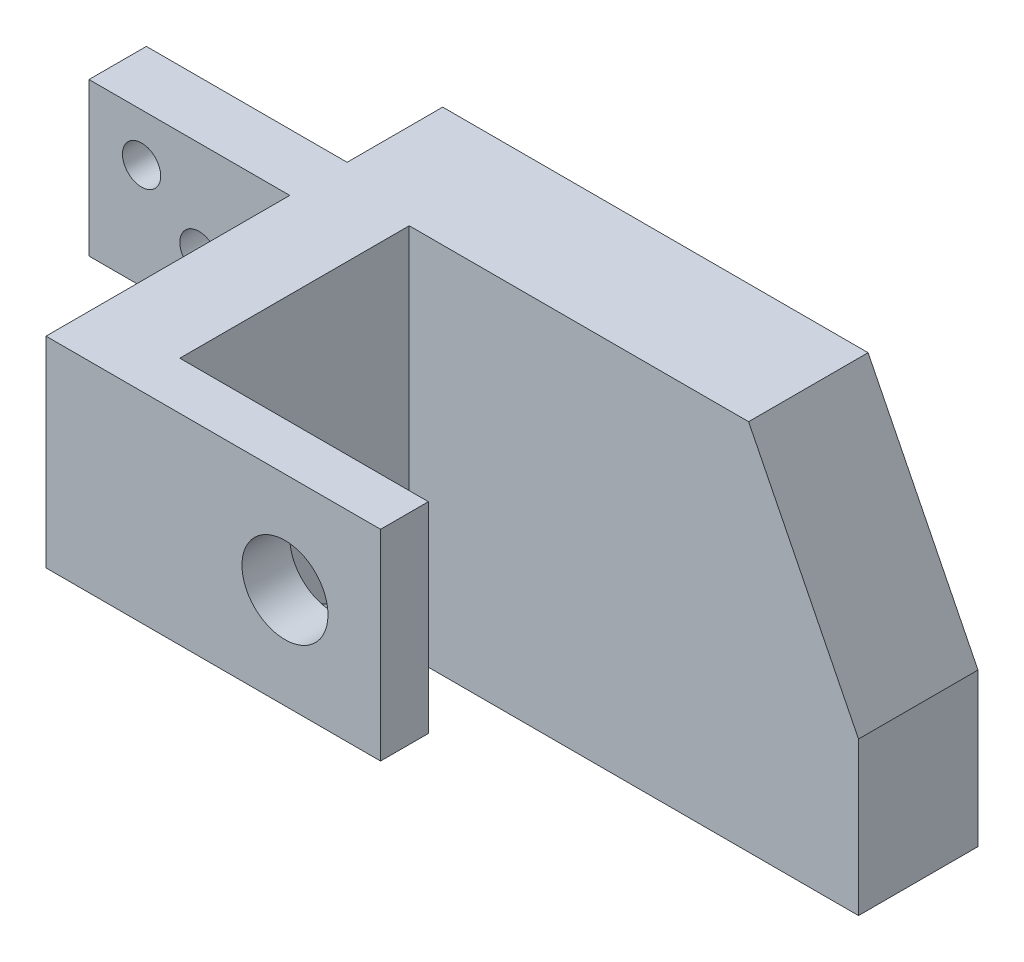
ISO-10303-21;
HEADER;
FILE_DESCRIPTION(('STEP AP214'),'2;1');
FILE_NAME('part.step','',(''),(''),'','','');
FILE_SCHEMA(('AUTOMOTIVE_DESIGN { 1 0 10303 214 1 1 1 1 }'));
ENDSEC;
DATA;
#1=APPLICATION_CONTEXT('core data for automotive mechanical design processes');
#2=APPLICATION_PROTOCOL_DEFINITION('international standard','automotive_design',2000,#1);
#3=PRODUCT_CONTEXT('',#1,'mechanical');
#4=PRODUCT('Part','Part','',(#3));
#5=PRODUCT_RELATED_PRODUCT_CATEGORY('part','',(#4));
#6=PRODUCT_DEFINITION_FORMATION('','',#4);
#7=PRODUCT_DEFINITION_CONTEXT('part definition',#1,'design');
#8=PRODUCT_DEFINITION('design','',#6,#7);
#9=PRODUCT_DEFINITION_SHAPE('','',#8);
#10=(LENGTH_UNIT() NAMED_UNIT(*) SI_UNIT(.MILLI.,.METRE.));
#11=(NAMED_UNIT(*) PLANE_ANGLE_UNIT() SI_UNIT($,.RADIAN.));
#12=(NAMED_UNIT(*) SI_UNIT($,.STERADIAN.) SOLID_ANGLE_UNIT());
#13=UNCERTAINTY_MEASURE_WITH_UNIT(LENGTH_MEASURE(1.E-05),#10,'distance_accuracy_value','');
#14=(GEOMETRIC_REPRESENTATION_CONTEXT(3) GLOBAL_UNCERTAINTY_ASSIGNED_CONTEXT((#13)) GLOBAL_UNIT_ASSIGNED_CONTEXT((#10,
#11,#12)) REPRESENTATION_CONTEXT('',''));
#15=CARTESIAN_POINT('',(0.,0.,0.));
#16=DIRECTION('',(0.,0.,1.));
#17=DIRECTION('',(1.,0.,0.));
#18=AXIS2_PLACEMENT_3D('',#15,#16,#17);
#19=CARTESIAN_POINT('',(0.,0.,25.));
#20=DIRECTION('',(1.,0.,0.));
#21=DIRECTION('',(0.,0.,-1.));
#22=AXIS2_PLACEMENT_3D('',#19,#20,#21);
#23=PLANE('',#22);
#24=DIRECTION('',(0.,-1.,0.));
#25=VECTOR('',#24,1.);
#26=CARTESIAN_POINT('',(0.,0.,25.));
#27=LINE('',#26,#25);
#28=CARTESIAN_POINT('',(0.,7.99999999999999,25.));
#29=VERTEX_POINT('',#28);
#30=CARTESIAN_POINT('',(0.,0.,25.));
#31=VERTEX_POINT('',#30);
#32=EDGE_CURVE('E254',#29,#31,#27,.T.);
#33=ORIENTED_EDGE('',*,*,#32,.F.);
#34=DIRECTION('',(0.,0.503871025524086,0.863778900898433));
#35=VECTOR('',#34,1.);
#36=CARTESIAN_POINT('',(0.,7.99999999999999,25.));
#37=LINE('',#36,#35);
#38=CARTESIAN_POINT('',(0.,36.,73.));
#39=VERTEX_POINT('',#38);
#40=EDGE_CURVE('E177',#29,#39,#37,.T.);
#41=ORIENTED_EDGE('',*,*,#40,.T.);
#42=DIRECTION('',(0.,0.,1.));
#43=VECTOR('',#42,1.);
#44=CARTESIAN_POINT('',(0.,36.,83.));
#45=LINE('',#44,#43);
#46=CARTESIAN_POINT('',(0.,36.,83.));
#47=VERTEX_POINT('',#46);
#48=EDGE_CURVE('E175',#39,#47,#45,.T.);
#49=ORIENTED_EDGE('',*,*,#48,.T.);
#50=DIRECTION('',(0.,1.,0.));
#51=VECTOR('',#50,1.);
#52=CARTESIAN_POINT('',(0.,78.,83.));
#53=LINE('',#52,#51);
#54=CARTESIAN_POINT('',(0.,78.,83.));
#55=VERTEX_POINT('',#54);
#56=EDGE_CURVE('E245',#47,#55,#53,.T.);
#57=ORIENTED_EDGE('',*,*,#56,.T.);
#58=DIRECTION('',(0.,0.,-1.));
#59=VECTOR('',#58,1.);
#60=CARTESIAN_POINT('',(0.,78.,25.));
#61=LINE('',#60,#59);
#62=CARTESIAN_POINT('',(0.,78.,32.));
#63=VERTEX_POINT('',#62);
#64=EDGE_CURVE('E273',#55,#63,#61,.T.);
#65=ORIENTED_EDGE('',*,*,#64,.T.);
#66=DIRECTION('',(0.,1.,0.));
#67=VECTOR('',#66,1.);
#68=CARTESIAN_POINT('',(0.,46.,32.));
#69=LINE('',#68,#67);
#70=CARTESIAN_POINT('',(0.,46.,32.));
#71=VERTEX_POINT('',#70);
#72=EDGE_CURVE('E218',#71,#63,#69,.T.);
#73=ORIENTED_EDGE('',*,*,#72,.F.);
#74=DIRECTION('',(0.,0.,1.));
#75=VECTOR('',#74,1.);
#76=CARTESIAN_POINT('',(0.,46.,20.));
#77=LINE('',#76,#75);
#78=CARTESIAN_POINT('',(0.,46.,20.));
#79=VERTEX_POINT('',#78);
#80=EDGE_CURVE('E223',#79,#71,#77,.T.);
#81=ORIENTED_EDGE('',*,*,#80,.F.);
#82=DIRECTION('',(0.,-1.,0.));
#83=VECTOR('',#82,1.);
#84=CARTESIAN_POINT('',(0.,78.,20.));
#85=LINE('',#84,#83);
#86=CARTESIAN_POINT('',(0.,78.,20.));
#87=VERTEX_POINT('',#86);
#88=EDGE_CURVE('E208',#87,#79,#85,.T.);
#89=ORIENTED_EDGE('',*,*,#88,.F.);
#90=CARTESIAN_POINT('',(0.,78.,0.));
#91=VERTEX_POINT('',#90);
#92=EDGE_CURVE('E264',#87,#91,#61,.T.);
#93=ORIENTED_EDGE('',*,*,#92,.T.);
#94=DIRECTION('',(0.,-1.,0.));
#95=VECTOR('',#94,1.);
#96=CARTESIAN_POINT('',(0.,0.,0.));
#97=LINE('',#96,#95);
#98=CARTESIAN_POINT('',(0.,0.,0.));
#99=VERTEX_POINT('',#98);
#100=EDGE_CURVE('E252',#91,#99,#97,.T.);
#101=ORIENTED_EDGE('',*,*,#100,.T.);
#102=DIRECTION('',(0.,0.,-1.));
#103=VECTOR('',#102,1.);
#104=CARTESIAN_POINT('',(0.,0.,25.));
#105=LINE('',#104,#103);
#106=EDGE_CURVE('E11',#31,#99,#105,.T.);
#107=ORIENTED_EDGE('',*,*,#106,.F.);
#108=EDGE_LOOP('',(#33,#41,#49,#57,#65,#73,#81,#89,#93,#101,#107));
#109=FACE_BOUND('',#108,.T.);
#110=ADVANCED_FACE('F44',(#109),#23,.F.);
#111=CARTESIAN_POINT('',(0.,0.,25.));
#112=DIRECTION('',(0.,1.,0.));
#113=DIRECTION('',(0.,0.,1.));
#114=AXIS2_PLACEMENT_3D('',#111,#112,#113);
#115=PLANE('',#114);
#116=DIRECTION('',(1.,0.,0.));
#117=VECTOR('',#116,1.);
#118=CARTESIAN_POINT('',(0.,0.,0.));
#119=LINE('',#118,#117);
#120=CARTESIAN_POINT('',(112.,0.,0.));
#121=VERTEX_POINT('',#120);
#122=EDGE_CURVE('E270',#99,#121,#119,.T.);
#123=ORIENTED_EDGE('',*,*,#122,.T.);
#124=DIRECTION('',(0.,0.,-1.));
#125=VECTOR('',#124,1.);
#126=CARTESIAN_POINT('',(112.,0.,25.));
#127=LINE('',#126,#125);
#128=CARTESIAN_POINT('',(112.,0.,25.));
#129=VERTEX_POINT('',#128);
#130=EDGE_CURVE('E55',#129,#121,#127,.T.);
#131=ORIENTED_EDGE('',*,*,#130,.F.);
#132=DIRECTION('',(1.,0.,0.));
#133=VECTOR('',#132,1.);
#134=CARTESIAN_POINT('',(0.,0.,25.));
#135=LINE('',#134,#133);
#136=EDGE_CURVE('E253',#31,#129,#135,.T.);
#137=ORIENTED_EDGE('',*,*,#136,.F.);
#138=ORIENTED_EDGE('',*,*,#106,.T.);
#139=EDGE_LOOP('',(#123,#131,#137,#138));
#140=FACE_BOUND('',#139,.T.);
#141=ADVANCED_FACE('F306',(#140),#115,.F.);
#142=CARTESIAN_POINT('',(112.,0.,25.));
#143=DIRECTION('',(-1.,0.,0.));
#144=DIRECTION('',(0.,0.,1.));
#145=AXIS2_PLACEMENT_3D('',#142,#143,#144);
#146=PLANE('',#145);
#147=DIRECTION('',(0.,1.,0.));
#148=VECTOR('',#147,1.);
#149=CARTESIAN_POINT('',(112.,0.,0.));
#150=LINE('',#149,#148);
#151=CARTESIAN_POINT('',(112.,32.,0.));
#152=VERTEX_POINT('',#151);
#153=EDGE_CURVE('E266',#121,#152,#150,.T.);
#154=ORIENTED_EDGE('',*,*,#153,.T.);
#155=DIRECTION('',(0.,0.,-1.));
#156=VECTOR('',#155,1.);
#157=CARTESIAN_POINT('',(112.,32.,25.));
#158=LINE('',#157,#156);
#159=CARTESIAN_POINT('',(112.,32.,25.));
#160=VERTEX_POINT('',#159);
#161=EDGE_CURVE('E278',#160,#152,#158,.T.);
#162=ORIENTED_EDGE('',*,*,#161,.F.);
#163=DIRECTION('',(0.,1.,0.));
#164=VECTOR('',#163,1.);
#165=CARTESIAN_POINT('',(112.,0.,25.));
#166=LINE('',#165,#164);
#167=EDGE_CURVE('E259',#129,#160,#166,.T.);
#168=ORIENTED_EDGE('',*,*,#167,.F.);
#169=ORIENTED_EDGE('',*,*,#130,.T.);
#170=EDGE_LOOP('',(#154,#162,#168,#169));
#171=FACE_BOUND('',#170,.T.);
#172=ADVANCED_FACE('F290',(#171),#146,.F.);
#173=CARTESIAN_POINT('',(89.,78.,25.));
#174=DIRECTION('',(-0.894427190999916,-0.447213595499958,0.));
#175=DIRECTION('',(0.447213595499958,-0.894427190999916,0.));
#176=AXIS2_PLACEMENT_3D('',#173,#174,#175);
#177=PLANE('',#176);
#178=DIRECTION('',(-0.447213595499958,0.894427190999916,0.));
#179=VECTOR('',#178,1.);
#180=CARTESIAN_POINT('',(89.,78.,0.));
#181=LINE('',#180,#179);
#182=CARTESIAN_POINT('',(89.,78.,0.));
#183=VERTEX_POINT('',#182);
#184=EDGE_CURVE('E272',#152,#183,#181,.T.);
#185=ORIENTED_EDGE('',*,*,#184,.T.);
#186=DIRECTION('',(0.,0.,-1.));
#187=VECTOR('',#186,1.);
#188=CARTESIAN_POINT('',(89.,78.,25.));
#189=LINE('',#188,#187);
#190=CARTESIAN_POINT('',(89.,78.,25.));
#191=VERTEX_POINT('',#190);
#192=EDGE_CURVE('E280',#191,#183,#189,.T.);
#193=ORIENTED_EDGE('',*,*,#192,.F.);
#194=DIRECTION('',(-0.447213595499958,0.894427190999916,0.));
#195=VECTOR('',#194,1.);
#196=CARTESIAN_POINT('',(89.,78.,25.));
#197=LINE('',#196,#195);
#198=EDGE_CURVE('E258',#160,#191,#197,.T.);
#199=ORIENTED_EDGE('',*,*,#198,.F.);
#200=ORIENTED_EDGE('',*,*,#161,.T.);
#201=EDGE_LOOP('',(#185,#193,#199,#200));
#202=FACE_BOUND('',#201,.T.);
#203=ADVANCED_FACE('F296',(#202),#177,.F.);
#204=CARTESIAN_POINT('',(0.,78.,25.));
#205=DIRECTION('',(0.,-1.,0.));
#206=DIRECTION('',(0.,0.,-1.));
#207=AXIS2_PLACEMENT_3D('',#204,#205,#206);
#208=PLANE('',#207);
#209=DIRECTION('',(-1.,0.,0.));
#210=VECTOR('',#209,1.);
#211=CARTESIAN_POINT('',(0.,78.,0.));
#212=LINE('',#211,#210);
#213=EDGE_CURVE('E257',#183,#91,#212,.T.);
#214=ORIENTED_EDGE('',*,*,#213,.T.);
#215=ORIENTED_EDGE('',*,*,#92,.F.);
#216=DIRECTION('',(1.,0.,0.));
#217=VECTOR('',#216,1.);
#218=CARTESIAN_POINT('',(-42.,78.,20.));
#219=LINE('',#218,#217);
#220=CARTESIAN_POINT('',(-42.,78.,20.));
#221=VERTEX_POINT('',#220);
#222=EDGE_CURVE('E238',#221,#87,#219,.T.);
#223=ORIENTED_EDGE('',*,*,#222,.F.);
#224=DIRECTION('',(0.,0.,-1.));
#225=VECTOR('',#224,1.);
#226=CARTESIAN_POINT('',(-42.,78.,32.));
#227=LINE('',#226,#225);
#228=CARTESIAN_POINT('',(-42.,78.,32.));
#229=VERTEX_POINT('',#228);
#230=EDGE_CURVE('E215',#229,#221,#227,.T.);
#231=ORIENTED_EDGE('',*,*,#230,.F.);
#232=DIRECTION('',(1.,0.,0.));
#233=VECTOR('',#232,1.);
#234=CARTESIAN_POINT('',(-42.,78.,32.));
#235=LINE('',#234,#233);
#236=EDGE_CURVE('E225',#229,#63,#235,.T.);
#237=ORIENTED_EDGE('',*,*,#236,.T.);
#238=ORIENTED_EDGE('',*,*,#64,.F.);
#239=DIRECTION('',(-1.,0.,0.));
#240=VECTOR('',#239,1.);
#241=CARTESIAN_POINT('',(18.,78.,83.));
#242=LINE('',#241,#240);
#243=CARTESIAN_POINT('',(70.,78.,83.));
#244=VERTEX_POINT('',#243);
#245=EDGE_CURVE('E247',#244,#55,#242,.T.);
#246=ORIENTED_EDGE('',*,*,#245,.F.);
#247=DIRECTION('',(0.,0.,1.));
#248=VECTOR('',#247,1.);
#249=CARTESIAN_POINT('',(70.,78.,73.));
#250=LINE('',#249,#248);
#251=CARTESIAN_POINT('',(70.,78.,73.));
#252=VERTEX_POINT('',#251);
#253=EDGE_CURVE('E210',#252,#244,#250,.T.);
#254=ORIENTED_EDGE('',*,*,#253,.F.);
#255=DIRECTION('',(-1.,0.,0.));
#256=VECTOR('',#255,1.);
#257=CARTESIAN_POINT('',(18.,78.,73.));
#258=LINE('',#257,#256);
#259=CARTESIAN_POINT('',(18.,78.,73.));
#260=VERTEX_POINT('',#259);
#261=EDGE_CURVE('E205',#252,#260,#258,.T.);
#262=ORIENTED_EDGE('',*,*,#261,.T.);
#263=DIRECTION('',(0.,0.,-1.));
#264=VECTOR('',#263,1.);
#265=CARTESIAN_POINT('',(18.,78.,25.));
#266=LINE('',#265,#264);
#267=CARTESIAN_POINT('',(18.,78.,25.));
#268=VERTEX_POINT('',#267);
#269=EDGE_CURVE('E155',#260,#268,#266,.T.);
#270=ORIENTED_EDGE('',*,*,#269,.T.);
#271=DIRECTION('',(-1.,0.,0.));
#272=VECTOR('',#271,1.);
#273=CARTESIAN_POINT('',(0.,78.,25.));
#274=LINE('',#273,#272);
#275=EDGE_CURVE('E265',#191,#268,#274,.T.);
#276=ORIENTED_EDGE('',*,*,#275,.F.);
#277=ORIENTED_EDGE('',*,*,#192,.T.);
#278=EDGE_LOOP('',(#214,#215,#223,#231,#237,#238,#246,#254,#262,#270,#276,#277));
#279=FACE_BOUND('',#278,.T.);
#280=ADVANCED_FACE('F305',(#279),#208,.F.);
#281=CARTESIAN_POINT('',(0.,0.,25.));
#282=DIRECTION('',(0.,0.,-1.));
#283=DIRECTION('',(-1.,0.,0.));
#284=AXIS2_PLACEMENT_3D('',#281,#282,#283);
#285=PLANE('',#284);
#286=DIRECTION('',(0.,-1.,0.));
#287=VECTOR('',#286,1.);
#288=CARTESIAN_POINT('',(18.,36.,25.));
#289=LINE('',#288,#287);
#290=CARTESIAN_POINT('',(18.,7.99999999999999,25.));
#291=VERTEX_POINT('',#290);
#292=EDGE_CURVE('E56',#268,#291,#289,.T.);
#293=ORIENTED_EDGE('',*,*,#292,.T.);
#294=DIRECTION('',(-1.,0.,0.));
#295=VECTOR('',#294,1.);
#296=CARTESIAN_POINT('',(18.,7.99999999999999,25.));
#297=LINE('',#296,#295);
#298=EDGE_CURVE('E64',#291,#29,#297,.T.);
#299=ORIENTED_EDGE('',*,*,#298,.T.);
#300=ORIENTED_EDGE('',*,*,#32,.T.);
#301=ORIENTED_EDGE('',*,*,#136,.T.);
#302=ORIENTED_EDGE('',*,*,#167,.T.);
#303=ORIENTED_EDGE('',*,*,#198,.T.);
#304=ORIENTED_EDGE('',*,*,#275,.T.);
#305=EDGE_LOOP('',(#293,#299,#300,#301,#302,#303,#304));
#306=FACE_BOUND('',#305,.T.);
#307=ADVANCED_FACE('F302',(#306),#285,.F.);
#308=CARTESIAN_POINT('',(0.,0.,0.));
#309=DIRECTION('',(0.,0.,-1.));
#310=DIRECTION('',(-1.,0.,0.));
#311=AXIS2_PLACEMENT_3D('',#308,#309,#310);
#312=PLANE('',#311);
#313=ORIENTED_EDGE('',*,*,#100,.F.);
#314=ORIENTED_EDGE('',*,*,#213,.F.);
#315=ORIENTED_EDGE('',*,*,#184,.F.);
#316=ORIENTED_EDGE('',*,*,#153,.F.);
#317=ORIENTED_EDGE('',*,*,#122,.F.);
#318=EDGE_LOOP('',(#313,#314,#315,#316,#317));
#319=FACE_BOUND('',#318,.T.);
#320=ADVANCED_FACE('F295',(#319),#312,.T.);
#321=CARTESIAN_POINT('',(18.,78.,83.));
#322=DIRECTION('',(0.,0.,1.));
#323=DIRECTION('',(1.,0.,0.));
#324=AXIS2_PLACEMENT_3D('',#321,#322,#323);
#325=PLANE('',#324);
#326=CARTESIAN_POINT('',(50.,57.,83.));
#327=DIRECTION('',(0.,0.,1.));
#328=DIRECTION('',(1.,0.,0.));
#329=AXIS2_PLACEMENT_3D('',#326,#327,#328);
#330=CIRCLE('',#329,9.);
#331=CARTESIAN_POINT('',(59.,57.,83.));
#332=VERTEX_POINT('',#331);
#333=EDGE_CURVE('E190',#332,#332,#330,.T.);
#334=ORIENTED_EDGE('',*,*,#333,.F.);
#335=EDGE_LOOP('',(#334));
#336=FACE_BOUND('',#335,.T.);
#337=ORIENTED_EDGE('',*,*,#56,.F.);
#338=DIRECTION('',(-1.,0.,0.));
#339=VECTOR('',#338,1.);
#340=CARTESIAN_POINT('',(18.,36.,83.));
#341=LINE('',#340,#339);
#342=CARTESIAN_POINT('',(70.,36.,83.));
#343=VERTEX_POINT('',#342);
#344=EDGE_CURVE('E242',#343,#47,#341,.T.);
#345=ORIENTED_EDGE('',*,*,#344,.F.);
#346=DIRECTION('',(0.,1.,0.));
#347=VECTOR('',#346,1.);
#348=CARTESIAN_POINT('',(70.,78.,83.));
#349=LINE('',#348,#347);
#350=EDGE_CURVE('E160',#343,#244,#349,.T.);
#351=ORIENTED_EDGE('',*,*,#350,.T.);
#352=ORIENTED_EDGE('',*,*,#245,.T.);
#353=EDGE_LOOP('',(#337,#345,#351,#352));
#354=FACE_BOUND('',#353,.T.);
#355=ADVANCED_FACE('F346',(#336,#354),#325,.T.);
#356=CARTESIAN_POINT('',(18.,36.,83.));
#357=DIRECTION('',(0.,-1.,0.));
#358=DIRECTION('',(0.,0.,-1.));
#359=AXIS2_PLACEMENT_3D('',#356,#357,#358);
#360=PLANE('',#359);
#361=DIRECTION('',(-1.,0.,0.));
#362=VECTOR('',#361,1.);
#363=CARTESIAN_POINT('',(18.,36.,73.));
#364=LINE('',#363,#362);
#365=CARTESIAN_POINT('',(18.,36.,73.));
#366=VERTEX_POINT('',#365);
#367=EDGE_CURVE('E169',#366,#39,#364,.T.);
#368=ORIENTED_EDGE('',*,*,#367,.F.);
#369=DIRECTION('',(1.,0.,0.));
#370=VECTOR('',#369,1.);
#371=CARTESIAN_POINT('',(70.,36.,73.));
#372=LINE('',#371,#370);
#373=CARTESIAN_POINT('',(70.,36.,73.));
#374=VERTEX_POINT('',#373);
#375=EDGE_CURVE('E157',#366,#374,#372,.T.);
#376=ORIENTED_EDGE('',*,*,#375,.T.);
#377=DIRECTION('',(0.,0.,1.));
#378=VECTOR('',#377,1.);
#379=CARTESIAN_POINT('',(70.,36.,73.));
#380=LINE('',#379,#378);
#381=EDGE_CURVE('E201',#374,#343,#380,.T.);
#382=ORIENTED_EDGE('',*,*,#381,.T.);
#383=ORIENTED_EDGE('',*,*,#344,.T.);
#384=ORIENTED_EDGE('',*,*,#48,.F.);
#385=EDGE_LOOP('',(#368,#376,#382,#383,#384));
#386=FACE_BOUND('',#385,.T.);
#387=ADVANCED_FACE('F167',(#386),#360,.T.);
#388=CARTESIAN_POINT('',(18.,0.,0.));
#389=DIRECTION('',(1.,0.,0.));
#390=DIRECTION('',(0.,0.,-1.));
#391=AXIS2_PLACEMENT_3D('',#388,#389,#390);
#392=PLANE('',#391);
#393=DIRECTION('',(0.,-1.,0.));
#394=VECTOR('',#393,1.);
#395=CARTESIAN_POINT('',(18.,36.,73.));
#396=LINE('',#395,#394);
#397=EDGE_CURVE('E150',#260,#366,#396,.T.);
#398=ORIENTED_EDGE('',*,*,#397,.T.);
#399=DIRECTION('',(0.,0.503871025524086,0.863778900898433));
#400=VECTOR('',#399,1.);
#401=CARTESIAN_POINT('',(18.,7.99999999999999,25.));
#402=LINE('',#401,#400);
#403=EDGE_CURVE('E153',#291,#366,#402,.T.);
#404=ORIENTED_EDGE('',*,*,#403,.F.);
#405=ORIENTED_EDGE('',*,*,#292,.F.);
#406=ORIENTED_EDGE('',*,*,#269,.F.);
#407=EDGE_LOOP('',(#398,#404,#405,#406));
#408=FACE_BOUND('',#407,.T.);
#409=ADVANCED_FACE('F146',(#408),#392,.T.);
#410=CARTESIAN_POINT('',(-42.,78.,20.));
#411=DIRECTION('',(0.,0.,1.));
#412=DIRECTION('',(1.,0.,0.));
#413=AXIS2_PLACEMENT_3D('',#410,#411,#412);
#414=PLANE('',#413);
#415=CARTESIAN_POINT('',(-31.,68.,20.));
#416=DIRECTION('',(0.,0.,1.));
#417=DIRECTION('',(1.,0.,0.));
#418=AXIS2_PLACEMENT_3D('',#415,#416,#417);
#419=CIRCLE('',#418,4.);
#420=CARTESIAN_POINT('',(-27.,68.,20.));
#421=VERTEX_POINT('',#420);
#422=EDGE_CURVE('E183',#421,#421,#419,.T.);
#423=ORIENTED_EDGE('',*,*,#422,.T.);
#424=EDGE_LOOP('',(#423));
#425=FACE_BOUND('',#424,.T.);
#426=CARTESIAN_POINT('',(-19.,58.,20.));
#427=DIRECTION('',(0.,0.,1.));
#428=DIRECTION('',(1.,0.,0.));
#429=AXIS2_PLACEMENT_3D('',#426,#427,#428);
#430=CIRCLE('',#429,4.);
#431=CARTESIAN_POINT('',(-15.,58.,20.));
#432=VERTEX_POINT('',#431);
#433=EDGE_CURVE('E192',#432,#432,#430,.T.);
#434=ORIENTED_EDGE('',*,*,#433,.T.);
#435=EDGE_LOOP('',(#434));
#436=FACE_BOUND('',#435,.T.);
#437=ORIENTED_EDGE('',*,*,#88,.T.);
#438=DIRECTION('',(1.,0.,0.));
#439=VECTOR('',#438,1.);
#440=CARTESIAN_POINT('',(-42.,46.,20.));
#441=LINE('',#440,#439);
#442=CARTESIAN_POINT('',(-42.,46.,20.));
#443=VERTEX_POINT('',#442);
#444=EDGE_CURVE('E232',#443,#79,#441,.T.);
#445=ORIENTED_EDGE('',*,*,#444,.F.);
#446=DIRECTION('',(0.,-1.,0.));
#447=VECTOR('',#446,1.);
#448=CARTESIAN_POINT('',(-42.,78.,20.));
#449=LINE('',#448,#447);
#450=EDGE_CURVE('E213',#221,#443,#449,.T.);
#451=ORIENTED_EDGE('',*,*,#450,.F.);
#452=ORIENTED_EDGE('',*,*,#222,.T.);
#453=EDGE_LOOP('',(#437,#445,#451,#452));
#454=FACE_BOUND('',#453,.T.);
#455=ADVANCED_FACE('F311',(#425,#436,#454),#414,.F.);
#456=CARTESIAN_POINT('',(-42.,46.,20.));
#457=DIRECTION('',(0.,1.,0.));
#458=DIRECTION('',(0.,0.,1.));
#459=AXIS2_PLACEMENT_3D('',#456,#457,#458);
#460=PLANE('',#459);
#461=ORIENTED_EDGE('',*,*,#80,.T.);
#462=DIRECTION('',(1.,0.,0.));
#463=VECTOR('',#462,1.);
#464=CARTESIAN_POINT('',(-42.,46.,32.));
#465=LINE('',#464,#463);
#466=CARTESIAN_POINT('',(-42.,46.,32.));
#467=VERTEX_POINT('',#466);
#468=EDGE_CURVE('E235',#467,#71,#465,.T.);
#469=ORIENTED_EDGE('',*,*,#468,.F.);
#470=DIRECTION('',(0.,0.,1.));
#471=VECTOR('',#470,1.);
#472=CARTESIAN_POINT('',(-42.,46.,20.));
#473=LINE('',#472,#471);
#474=EDGE_CURVE('E216',#443,#467,#473,.T.);
#475=ORIENTED_EDGE('',*,*,#474,.F.);
#476=ORIENTED_EDGE('',*,*,#444,.T.);
#477=EDGE_LOOP('',(#461,#469,#475,#476));
#478=FACE_BOUND('',#477,.T.);
#479=ADVANCED_FACE('F325',(#478),#460,.F.);
#480=CARTESIAN_POINT('',(-42.,46.,32.));
#481=DIRECTION('',(0.,0.,-1.));
#482=DIRECTION('',(0.,1.,0.));
#483=AXIS2_PLACEMENT_3D('',#480,#481,#482);
#484=PLANE('',#483);
#485=CARTESIAN_POINT('',(-31.,68.,32.));
#486=DIRECTION('',(0.,0.,1.));
#487=DIRECTION('',(1.,0.,0.));
#488=AXIS2_PLACEMENT_3D('',#485,#486,#487);
#489=CIRCLE('',#488,4.);
#490=CARTESIAN_POINT('',(-27.,68.,32.));
#491=VERTEX_POINT('',#490);
#492=EDGE_CURVE('E189',#491,#491,#489,.T.);
#493=ORIENTED_EDGE('',*,*,#492,.F.);
#494=EDGE_LOOP('',(#493));
#495=FACE_BOUND('',#494,.T.);
#496=CARTESIAN_POINT('',(-19.,58.,32.));
#497=DIRECTION('',(0.,0.,1.));
#498=DIRECTION('',(1.,0.,0.));
#499=AXIS2_PLACEMENT_3D('',#496,#497,#498);
#500=CIRCLE('',#499,4.);
#501=CARTESIAN_POINT('',(-15.,58.,32.));
#502=VERTEX_POINT('',#501);
#503=EDGE_CURVE('E176',#502,#502,#500,.T.);
#504=ORIENTED_EDGE('',*,*,#503,.F.);
#505=EDGE_LOOP('',(#504));
#506=FACE_BOUND('',#505,.T.);
#507=ORIENTED_EDGE('',*,*,#72,.T.);
#508=ORIENTED_EDGE('',*,*,#236,.F.);
#509=DIRECTION('',(0.,1.,0.));
#510=VECTOR('',#509,1.);
#511=CARTESIAN_POINT('',(-42.,46.,32.));
#512=LINE('',#511,#510);
#513=EDGE_CURVE('E217',#467,#229,#512,.T.);
#514=ORIENTED_EDGE('',*,*,#513,.F.);
#515=ORIENTED_EDGE('',*,*,#468,.T.);
#516=EDGE_LOOP('',(#507,#508,#514,#515));
#517=FACE_BOUND('',#516,.T.);
#518=ADVANCED_FACE('F316',(#495,#506,#517),#484,.F.);
#519=CARTESIAN_POINT('',(-42.,0.,0.));
#520=DIRECTION('',(-1.,0.,0.));
#521=DIRECTION('',(0.,0.,1.));
#522=AXIS2_PLACEMENT_3D('',#519,#520,#521);
#523=PLANE('',#522);
#524=ORIENTED_EDGE('',*,*,#230,.T.);
#525=ORIENTED_EDGE('',*,*,#450,.T.);
#526=ORIENTED_EDGE('',*,*,#474,.T.);
#527=ORIENTED_EDGE('',*,*,#513,.T.);
#528=EDGE_LOOP('',(#524,#525,#526,#527));
#529=FACE_BOUND('',#528,.T.);
#530=ADVANCED_FACE('F314',(#529),#523,.T.);
#531=CARTESIAN_POINT('',(70.,78.,73.));
#532=DIRECTION('',(1.,0.,0.));
#533=DIRECTION('',(0.,0.,-1.));
#534=AXIS2_PLACEMENT_3D('',#531,#532,#533);
#535=PLANE('',#534);
#536=ORIENTED_EDGE('',*,*,#350,.F.);
#537=ORIENTED_EDGE('',*,*,#381,.F.);
#538=DIRECTION('',(0.,1.,0.));
#539=VECTOR('',#538,1.);
#540=CARTESIAN_POINT('',(70.,78.,73.));
#541=LINE('',#540,#539);
#542=EDGE_CURVE('E165',#374,#252,#541,.T.);
#543=ORIENTED_EDGE('',*,*,#542,.T.);
#544=ORIENTED_EDGE('',*,*,#253,.T.);
#545=EDGE_LOOP('',(#536,#537,#543,#544));
#546=FACE_BOUND('',#545,.T.);
#547=ADVANCED_FACE('F390',(#546),#535,.T.);
#548=CARTESIAN_POINT('',(0.,0.,73.));
#549=DIRECTION('',(0.,0.,-1.));
#550=DIRECTION('',(-1.,0.,0.));
#551=AXIS2_PLACEMENT_3D('',#548,#549,#550);
#552=PLANE('',#551);
#553=CARTESIAN_POINT('',(50.,57.,73.));
#554=DIRECTION('',(0.,0.,1.));
#555=DIRECTION('',(1.,0.,0.));
#556=AXIS2_PLACEMENT_3D('',#553,#554,#555);
#557=CIRCLE('',#556,9.);
#558=CARTESIAN_POINT('',(59.,57.,73.));
#559=VERTEX_POINT('',#558);
#560=EDGE_CURVE('E198',#559,#559,#557,.T.);
#561=ORIENTED_EDGE('',*,*,#560,.T.);
#562=EDGE_LOOP('',(#561));
#563=FACE_BOUND('',#562,.T.);
#564=ORIENTED_EDGE('',*,*,#397,.F.);
#565=ORIENTED_EDGE('',*,*,#261,.F.);
#566=ORIENTED_EDGE('',*,*,#542,.F.);
#567=ORIENTED_EDGE('',*,*,#375,.F.);
#568=EDGE_LOOP('',(#564,#565,#566,#567));
#569=FACE_BOUND('',#568,.T.);
#570=ADVANCED_FACE('F162',(#563,#569),#552,.T.);
#571=CARTESIAN_POINT('',(50.,57.,73.));
#572=DIRECTION('',(0.,0.,1.));
#573=DIRECTION('',(1.,0.,0.));
#574=AXIS2_PLACEMENT_3D('',#571,#572,#573);
#575=CYLINDRICAL_SURFACE('',#574,9.);
#576=ORIENTED_EDGE('',*,*,#560,.F.);
#577=EDGE_LOOP('',(#576));
#578=FACE_BOUND('',#577,.T.);
#579=ORIENTED_EDGE('',*,*,#333,.T.);
#580=EDGE_LOOP('',(#579));
#581=FACE_BOUND('',#580,.T.);
#582=ADVANCED_FACE('F394',(#578,#581),#575,.F.);
#583=CARTESIAN_POINT('',(-19.,58.,20.));
#584=DIRECTION('',(0.,0.,1.));
#585=DIRECTION('',(1.,0.,0.));
#586=AXIS2_PLACEMENT_3D('',#583,#584,#585);
#587=CYLINDRICAL_SURFACE('',#586,4.);
#588=ORIENTED_EDGE('',*,*,#433,.F.);
#589=EDGE_LOOP('',(#588));
#590=FACE_BOUND('',#589,.T.);
#591=ORIENTED_EDGE('',*,*,#503,.T.);
#592=EDGE_LOOP('',(#591));
#593=FACE_BOUND('',#592,.T.);
#594=ADVANCED_FACE('F399',(#590,#593),#587,.F.);
#595=CARTESIAN_POINT('',(-31.,68.,20.));
#596=DIRECTION('',(0.,0.,1.));
#597=DIRECTION('',(1.,0.,0.));
#598=AXIS2_PLACEMENT_3D('',#595,#596,#597);
#599=CYLINDRICAL_SURFACE('',#598,4.);
#600=ORIENTED_EDGE('',*,*,#422,.F.);
#601=EDGE_LOOP('',(#600));
#602=FACE_BOUND('',#601,.T.);
#603=ORIENTED_EDGE('',*,*,#492,.T.);
#604=EDGE_LOOP('',(#603));
#605=FACE_BOUND('',#604,.T.);
#606=ADVANCED_FACE('F410',(#602,#605),#599,.F.);
#607=CARTESIAN_POINT('',(18.,7.99999999999999,25.));
#608=DIRECTION('',(0.,-0.863778900898433,0.503871025524086));
#609=DIRECTION('',(0.,-0.503871025524086,-0.863778900898433));
#610=AXIS2_PLACEMENT_3D('',#607,#608,#609);
#611=PLANE('',#610);
#612=ORIENTED_EDGE('',*,*,#40,.F.);
#613=ORIENTED_EDGE('',*,*,#298,.F.);
#614=ORIENTED_EDGE('',*,*,#403,.T.);
#615=ORIENTED_EDGE('',*,*,#367,.T.);
#616=EDGE_LOOP('',(#612,#613,#614,#615));
#617=FACE_BOUND('',#616,.T.);
#618=ADVANCED_FACE('F178',(#617),#611,.T.);
#619=CLOSED_SHELL('',(#110,#141,#172,#203,#280,#307,#320,#355,#387,#409,#455,#479,#518,#530,
#547,#570,#582,#594,#606,#618));
#620=MANIFOLD_SOLID_BREP('B2',#619);
#621=ADVANCED_BREP_SHAPE_REPRESENTATION('',(#18,#620),#14);
#622=SHAPE_DEFINITION_REPRESENTATION(#9,#621);
ENDSEC;
END-ISO-10303-21;
